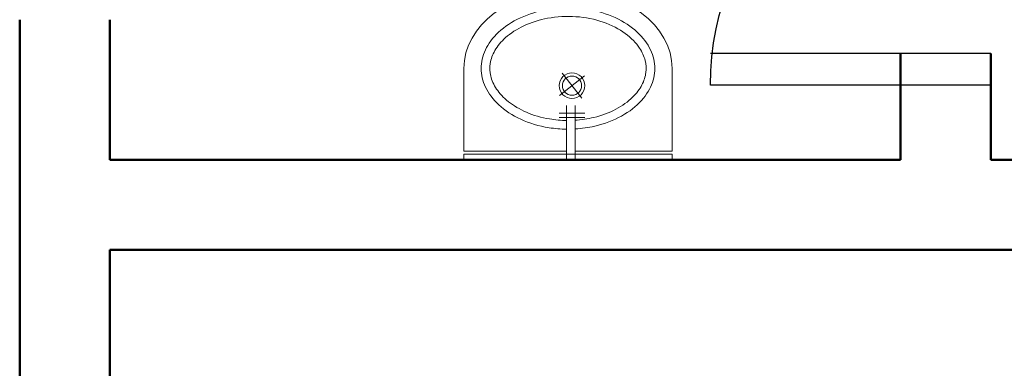
# Model space of a CAD drawing. Units: millimetres. Extents: x -857 to 54106, y -13666 to 13947.
# Tile 15 of 41: x 21020 to 23479, y 7433 to 8304. Entities that reach past the tile are written whole.
import ezdxf

# ---------------------------------------------------------------- set-up
doc = ezdxf.new("R2010")
doc.units = ezdxf.units.MM
for name, color, linetype, lineweight in [('A-DOOR', 1, 'Continuous', 25), ('A-FLOR-FIXT', 8, 'Continuous', 18), ('A-SANITARY FITTINGS', 25, 'Continuous', 15), ('A-WALL', 7, 'Continuous', 50)]:
    doc.layers.add(name, color=color, linetype=linetype, lineweight=lineweight)

# ---------------------------------------------------------------- blocks, each defined once
blk = doc.blocks.new('A$C0124305E')
at = {"layer": 'A-SANITARY FITTINGS'}
for p, q in [((-8.415, 16.014), (-0.8, 16.014)), ((-0.8, 7.082), (-0.8, 16.014)), ((-5.663, 7.684), (-7.996, 5.88)), ((-7.731, 7.949), (-5.927, 5.616)), ((-4.306, 5.613), (-4.306, 7.962)), ((-3.906, 5.613), (-3.906, 7.962)), ((0, 7.082), (-4.992, 7.082)), ((0, 6.282), (-4.992, 6.282)), ((-0.8, -3.186), (-0.8, 6.282)), ((-8.415, -3.186), (-0.8, -3.186))]:
    blk.add_line(p, q, dxfattribs=at)
blk.add_lwpolyline([(-0.5, 16.014), (0, 16.014), (0, -3.186), (-0.5, -3.186)], close=True, dxfattribs=at)
for radius in [1.18, 0.885]:
    blk.add_circle((-6.829, 6.782), radius, dxfattribs=at)
at = {"layer": 'A-SANITARY FITTINGS', "extrusion": (0, 0, -1)}
blk.add_ellipse((-8.415, 6.414), major_axis=(0, 9.6), ratio=0.75, start_param=3.141593, end_param=6.283185, dxfattribs=at)
at = {"layer": 'A-SANITARY FITTINGS'}
for points, knots in [([(-2.816, 6.282), (-2.822, 5.739), (-2.868, 5.198), (-3.101, 3.742), (-3.367, 2.857), (-4.09, 1.283), (-4.545, 0.595), (-5.561, -0.504), (-6.119, -0.915), (-7.254, -1.454), (-7.83, -1.584), (-8.977, -1.588), (-9.553, -1.461), (-10.689, -0.93), (-11.247, -0.523), (-12.266, 0.569), (-12.723, 1.253), (-13.451, 2.821), (-13.721, 3.705), (-14.023, 5.556), (-14.055, 6.522), (-13.877, 8.407), (-13.666, 9.325), (-13.039, 10.989), (-12.624, 11.735), (-11.665, 12.964), (-11.123, 13.448), (-10.003, 14.125), (-9.426, 14.322), (-8.279, 14.455), (-7.704, 14.392), (-6.561, 13.997), (-5.992, 13.662), (-4.929, 12.706), (-4.437, 12.086), (-3.622, 10.621), (-3.3, 9.776), (-2.958, 8.295), (-2.872, 7.691), (-2.835, 7.082)], [1.58652, 1.58652, 1.58652, 1.58652, 1.780321, 1.780321, 2.120053, 2.120053, 2.459785, 2.459785, 2.799517, 2.799517, 3.139249, 3.139249, 3.478981, 3.478981, 3.818713, 3.818713, 4.158445, 4.158445, 4.498177, 4.498177, 4.837909, 4.837909, 5.177641, 5.177641, 5.517373, 5.517373, 5.857105, 5.857105, 6.196837, 6.196837, 6.536569, 6.536569, 6.876301, 6.876301, 7.216033, 7.216033, 7.555765, 7.555765, 7.774364, 7.774364, 7.774364, 7.774364]), ([(-3.616, 6.291), (-3.622, 5.761), (-3.669, 5.23), (-3.883, 3.956), (-4.098, 3.227), (-4.649, 1.948), (-4.984, 1.391), (-5.718, 0.465), (-6.116, 0.099), (-6.921, -0.44), (-7.323, -0.613), (-8.109, -0.797), (-8.496, -0.811), (-9.278, -0.688), (-9.675, -0.549), (-10.48, -0.084), (-10.885, 0.244), (-11.669, 1.127), (-12.046, 1.699), (-12.659, 3.011), (-12.897, 3.755), (-13.201, 5.382), (-13.251, 6.275), (-13.128, 8.021), (-12.952, 8.877), (-12.417, 10.425), (-12.055, 11.118), (-11.23, 12.254), (-10.765, 12.696), (-9.915, 13.262), (-9.531, 13.429), (-8.777, 13.616), (-8.406, 13.637), (-7.66, 13.542), (-7.28, 13.424), (-6.51, 13.021), (-6.123, 12.734), (-5.353, 11.947), (-4.975, 11.432), (-4.338, 10.23), (-4.077, 9.541), (-3.76, 8.238), (-3.67, 7.639), (-3.634, 7.034)], [1.58652, 1.58652, 1.58652, 1.58652, 1.790653, 1.790653, 2.093007, 2.093007, 2.384527, 2.384527, 2.676047, 2.676047, 2.967567, 2.967567, 3.259087, 3.259087, 3.550608, 3.550608, 3.842128, 3.842128, 4.155456, 4.155456, 4.468784, 4.468784, 4.806699, 4.806699, 5.144614, 5.144614, 5.482529, 5.482529, 5.820444, 5.820444, 6.099515, 6.099515, 6.378586, 6.378586, 6.657656, 6.657656, 6.936727, 6.936727, 7.23864, 7.23864, 7.540552, 7.540552, 7.774364, 7.774364, 7.774364, 7.774364])]:
    blk.add_open_spline(points, degree=3, knots=knots, dxfattribs=at)
blk = doc.blocks.new('DOOR-700')
blk.add_line((8245.5, 10779.2), (8245.5, 11479.2))
blk.add_arc((8245.5, 10779.2), 700, 90, 180)

msp = doc.modelspace()

# ---------------------------------------------------------------- linework, layer by layer
at = {"layer": 'A-DOOR'}
for p, q in [((23445.079, 8220.088), (22745.079, 8220.088)), ((23445.079, 8140.088), (23445.079, 8220.088)), ((23445.079, 8140.088), (23445.079, 8220.088))]:
    msp.add_line(p, q, dxfattribs=at)
at = {"layer": 'A-WALL'}
for p, q in [((21245.079, 8304.231), (21245.079, 7954.231)), ((23220.079, 7954.231), (23220.079, 8220.088)), ((23445.079, 7954.231), (23445.079, 8220.088)), ((21245.079, 7954.231), (23220.079, 7954.231)), ((23584.957, 7954.231), (23445.079, 7954.231)), ((21245.079, 7729.231), (23613.536, 7729.231)), ((21245.079, 6467.586), (21245.079, 7729.231))]:
    msp.add_line(p, q, dxfattribs=at)
msp.add_lwpolyline([(21020.079, 6467.586), (21020.079, 8304.231)], dxfattribs=at)

# ---------------------------------------------------------------- block references
at = {"layer": 'A-DOOR', "extrusion": (0, 0, -1), "zscale": -1, "rotation": 269.9999999999999}
msp.add_blockref('DOOR-700', (-34224.31, 16385.634), dxfattribs=at)
at = {"layer": 'A-FLOR-FIXT', "xscale": 27.10344997005861, "yscale": 27.10344997005861, "zscale": 27.10344997005861, "rotation": 270.0000000004072}
msp.add_blockref('A$C0124305E', (22215.607, 7954.231), dxfattribs=at)

doc.saveas('drawing.dxf')
